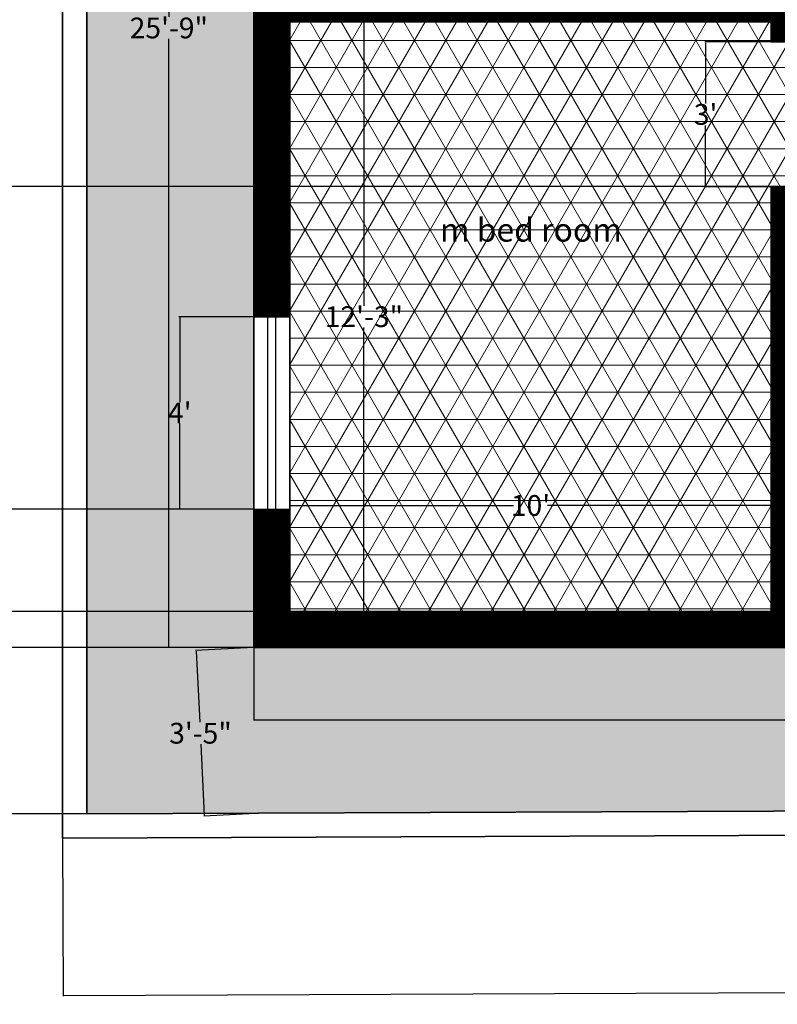
# Model space of a CAD drawing. Units: inches. Extents: x -157 to 1464, y -361 to 1077.
# Tile 3 of 9: x 241 to 430, y 23 to 268. Entities that reach past the tile are written whole.
import ezdxf

# ---------------------------------------------------------------- set-up
doc = ezdxf.new("R2010")
doc.units = ezdxf.units.IN
doc.header["$MEASUREMENT"] = 0
for name, color, linetype, lineweight in [('A-ANNO-DIMS', 2, 'Continuous', 18), ('A-AREA-IDEN', 7, 'Continuous', 18), ('A-FLOR-PATT', 8, 'Continuous', 13), ('A-WALL', 7, 'Continuous', 35), ('A-WALL-PATT', 252, 'Continuous', 13), ('C-ANNO-DIMS', 2, 'Continuous', 18), ('C-PROP', 7, 'Continuous', 35), ('doors and windows', 33, 'Continuous', 25), ('L-GRND-PATT', 8, 'Continuous', 13)]:
    doc.layers.add(name, color=color, linetype=linetype, lineweight=lineweight)
doc.styles.get("Standard").update_dxf_attribs({"font": 'arial.ttf'})
doc.dimstyles.new('Annotative', dxfattribs={"dimscale": 0, "dimtxt": 5.18, "dimasz": 0.18, "dimexe": 0.18, "dimexo": 0.0625, "dimgap": 0.09, "dimtad": 0, "dimtih": 1, "dimtoh": 1, "dimdec": 0, "dimzin": 0, "dimdsep": 46, "dimlunit": 3, "dimtxsty": 'Standard', "dimcen": 0.09, "dimadec": 0, "dimazin": 0, "dimtfac": 1, "dimtdec": 0, "dimtofl": 0, "dimtmove": 0, "dimatfit": 3, "dimfxl": 1, "dimtolj": 1, "dimtzin": 0, "dimarcsym": 0})

# ---------------------------------------------------------------- blocks, each defined once
blk = doc.blocks.new('*D1')
at = {"layer": 'A-ANNO-DIMS', "color": 0, "lineweight": -2, "transparency": 16777216}
for p, q in [((298.9, 420.86), (277.62, 420.86)), ((277.8, 420.68), (277.8, 269.1)), ((277.8, 112.04), (277.8, 263.63)), ((298.9, 111.86), (277.62, 111.86))]:
    blk.add_line(p, q, dxfattribs=at)
at = {"layer": 'A-ANNO-DIMS', "color": 0, "transparency": 16777216}
for points in [[(277.77, 420.68), (277.83, 420.68), (277.8, 420.86)], [(277.77, 112.04), (277.83, 112.04), (277.8, 111.86)]]:
    blk.add_solid(points, dxfattribs=at)
at = {"layer": 'Defpoints', "color": 0, "transparency": 16777216}
for p in [(298.97, 420.86), (277.8, 111.86), (298.97, 111.86)]:
    blk.add_point(p, dxfattribs=at)
at = {"layer": 'A-ANNO-DIMS', "color": 0, "transparency": 16777216, "insert": (277.8, 266.36), "char_height": 5.18, "attachment_point": 5}
blk.add_mtext('\\A1;25\'-9"', dxfattribs=at)
blk = doc.blocks.new('*D2')
at = {"layer": 'A-ANNO-DIMS', "color": 0, "lineweight": -2, "transparency": 16777216}
for p, q in [((298.97, 111.8), (298.97, 93.67)), ((596.97, 111.8), (596.97, 93.67)), ((299.15, 93.85), (436.92, 93.85)), ((596.79, 93.85), (459.01, 93.85))]:
    blk.add_line(p, q, dxfattribs=at)
at = {"layer": 'A-ANNO-DIMS', "color": 0, "transparency": 16777216}
for points in [[(299.15, 93.88), (299.15, 93.82), (298.97, 93.85)], [(596.79, 93.88), (596.79, 93.82), (596.97, 93.85)]]:
    blk.add_solid(points, dxfattribs=at)
at = {"layer": 'Defpoints', "color": 0, "transparency": 16777216}
for p in [(298.97, 111.86), (596.97, 111.86), (596.97, 93.85)]:
    blk.add_point(p, dxfattribs=at)
at = {"layer": 'A-ANNO-DIMS', "color": 0, "transparency": 16777216, "insert": (447.97, 93.85), "char_height": 5.18, "attachment_point": 5}
blk.add_mtext('\\A1;24\'-10"', dxfattribs=at)
blk = doc.blocks.new('*D3')
at = {"layer": 'A-ANNO-DIMS', "color": 0, "lineweight": -2, "transparency": 16777216}
for p, q in [((308.03, 267.86), (326.61, 267.86)), ((326.43, 267.68), (326.43, 197.1)), ((326.43, 121.04), (326.43, 191.62)), ((308.03, 120.86), (326.61, 120.86))]:
    blk.add_line(p, q, dxfattribs=at)
at = {"layer": 'A-ANNO-DIMS', "color": 0, "transparency": 16777216}
for points in [[(326.4, 267.68), (326.46, 267.68), (326.43, 267.86)], [(326.4, 121.04), (326.46, 121.04), (326.43, 120.86)]]:
    blk.add_solid(points, dxfattribs=at)
at = {"layer": 'Defpoints', "color": 0, "transparency": 16777216}
for p in [(307.97, 267.86), (307.97, 120.86), (326.43, 120.86)]:
    blk.add_point(p, dxfattribs=at)
at = {"layer": 'A-ANNO-DIMS', "color": 0, "transparency": 16777216, "insert": (326.43, 194.36), "char_height": 5.18, "attachment_point": 5}
blk.add_mtext('\\A1;12\'-3"', dxfattribs=at)
blk = doc.blocks.new('*D4')
at = {"layer": 'A-ANNO-DIMS', "color": 0, "lineweight": -2, "transparency": 16777216}
for p, q in [((307.97, 120.92), (307.97, 147.45)), ((427.97, 120.92), (427.97, 147.45)), ((308.15, 147.27), (363.72, 147.27)), ((427.79, 147.27), (372.21, 147.27))]:
    blk.add_line(p, q, dxfattribs=at)
at = {"layer": 'A-ANNO-DIMS', "color": 0, "transparency": 16777216}
for points in [[(308.15, 147.3), (308.15, 147.24), (307.97, 147.27)], [(427.79, 147.3), (427.79, 147.24), (427.97, 147.27)]]:
    blk.add_solid(points, dxfattribs=at)
at = {"layer": 'Defpoints', "color": 0, "transparency": 16777216}
for p in [(427.97, 147.27), (307.97, 120.86), (427.97, 120.86)]:
    blk.add_point(p, dxfattribs=at)
at = {"layer": 'A-ANNO-DIMS', "color": 0, "transparency": 16777216, "insert": (367.97, 147.27), "char_height": 5.18, "attachment_point": 5}
blk.add_mtext("\\A1;10'", dxfattribs=at)
blk = doc.blocks.new('*D13')
at = {"layer": 'C-ANNO-DIMS', "color": 0, "lineweight": -2, "transparency": 16777216}
for p, q in [((257.27, 643.42), (188.08, 643.42)), ((188.26, 643.24), (188.26, 359.63)), ((188.26, 70.55), (188.26, 354.16)), ((257.27, 70.37), (188.08, 70.37))]:
    blk.add_line(p, q, dxfattribs=at)
at = {"layer": 'C-ANNO-DIMS', "color": 0, "transparency": 16777216}
for points in [[(188.23, 643.24), (188.29, 643.24), (188.26, 643.42)], [(188.23, 70.55), (188.29, 70.55), (188.26, 70.37)]]:
    blk.add_solid(points, dxfattribs=at)
at = {"layer": 'Defpoints', "color": 0, "transparency": 16777216}
for p in [(257.33, 643.42), (188.26, 70.37), (257.33, 70.37)]:
    blk.add_point(p, dxfattribs=at)
at = {"layer": 'C-ANNO-DIMS', "color": 0, "transparency": 16777216, "insert": (188.26, 356.89), "char_height": 5.18, "attachment_point": 5}
blk.add_mtext('\\A1;47\'-9"', dxfattribs=at)
blk = doc.blocks.new('*D14')
at = {"layer": 'C-ANNO-DIMS', "color": 0, "lineweight": -2, "transparency": 16777216}
for p, q in [((862.57, 66.62), (862.72, 27.26)), ((251.33, 64.28), (251.48, 24.92)), ((862.54, 27.44), (568.1, 26.31)), ((251.66, 25.1), (546.1, 26.23))]:
    blk.add_line(p, q, dxfattribs=at)
at = {"layer": 'C-ANNO-DIMS', "color": 0, "transparency": 16777216}
for points in [[(862.54, 27.47), (862.54, 27.41), (862.72, 27.44)], [(251.66, 25.13), (251.66, 25.07), (251.48, 25.1)]]:
    blk.add_solid(points, dxfattribs=at)
at = {"layer": 'Defpoints', "color": 0, "transparency": 16777216}
for p in [(862.57, 66.68), (251.33, 64.34), (862.72, 27.44)]:
    blk.add_point(p, dxfattribs=at)
at = {"layer": 'C-ANNO-DIMS', "color": 0, "transparency": 16777216, "insert": (557.1, 26.27), "char_height": 5.18, "attachment_point": 5}
blk.add_mtext('\\A1;50\'-11"', dxfattribs=at)
blk = doc.blocks.new('*D28')
at = {"layer": 'A-ANNO-DIMS', "color": 0, "lineweight": -2, "transparency": 16777216}
for p, q in [((427.9, 262.86), (411.45, 262.86)), ((411.63, 262.68), (411.63, 247.54)), ((411.63, 226.92), (411.63, 242.06)), ((427.9, 226.74), (411.45, 226.74))]:
    blk.add_line(p, q, dxfattribs=at)
at = {"layer": 'A-ANNO-DIMS', "color": 0, "transparency": 16777216}
for points in [[(411.6, 262.68), (411.66, 262.68), (411.63, 262.86)], [(411.6, 226.92), (411.66, 226.92), (411.63, 226.74)]]:
    blk.add_solid(points, dxfattribs=at)
at = {"layer": 'Defpoints', "color": 0, "transparency": 16777216}
for p in [(427.97, 262.86), (411.63, 226.74), (427.97, 226.74)]:
    blk.add_point(p, dxfattribs=at)
at = {"layer": 'A-ANNO-DIMS', "color": 0, "transparency": 16777216, "insert": (411.63, 244.8), "char_height": 5.18, "attachment_point": 5}
blk.add_mtext("\\A1;3'", dxfattribs=at)
blk = doc.blocks.new('*D49')
at = {"layer": 'A-ANNO-DIMS', "color": 0, "lineweight": -2, "transparency": 16777216}
for p, q in [((298.9, 194.36), (280.34, 194.36)), ((280.52, 194.18), (280.52, 173.04)), ((280.52, 146.54), (280.52, 167.68)), ((298.9, 146.36), (280.34, 146.36))]:
    blk.add_line(p, q, dxfattribs=at)
at = {"layer": 'A-ANNO-DIMS', "color": 0, "transparency": 16777216}
for points in [[(280.49, 194.18), (280.55, 194.18), (280.52, 194.36)], [(280.49, 146.54), (280.55, 146.54), (280.52, 146.36)]]:
    blk.add_solid(points, dxfattribs=at)
at = {"layer": 'Defpoints', "color": 0, "transparency": 16777216}
for p in [(298.97, 194.36), (280.52, 146.36), (298.97, 146.36)]:
    blk.add_point(p, dxfattribs=at)
at = {"layer": 'A-ANNO-DIMS', "color": 0, "transparency": 16777216, "insert": (280.52, 170.36), "char_height": 5.18, "attachment_point": 5}
blk.add_mtext("\\A1;4'", dxfattribs=at)
blk = doc.blocks.new('*D54')
at = {"layer": 'C-ANNO-DIMS', "color": 0, "lineweight": -2, "transparency": 16777216}
for p, q in [((298.9, 111.86), (284.47, 111.13)), ((284.66, 110.96), (285.56, 93.21)), ((286.74, 69.99), (285.84, 87.73)), ((301, 70.53), (286.57, 69.8))]:
    blk.add_line(p, q, dxfattribs=at)
at = {"layer": 'C-ANNO-DIMS', "color": 0, "transparency": 16777216}
for points in [[(284.69, 110.96), (284.63, 110.95), (284.65, 111.14)], [(286.77, 69.99), (286.71, 69.99), (286.75, 69.81)]]:
    blk.add_solid(points, dxfattribs=at)
at = {"layer": 'Defpoints', "color": 0, "transparency": 16777216}
for p in [(298.97, 111.86), (286.75, 69.81), (301.06, 70.53)]:
    blk.add_point(p, dxfattribs=at)
at = {"layer": 'C-ANNO-DIMS', "color": 0, "transparency": 16777216, "insert": (285.7, 90.47), "char_height": 5.18, "attachment_point": 5}
blk.add_mtext('\\A1;3\'-5"', dxfattribs=at)
blk = doc.blocks.new('WIN-48x9')
for p, q in [((9, 48), (0, 48)), ((0, 48), (0, 0)), ((3.5, 48), (3.5, 0)), ((5.5, 48), (5.5, 0)), ((9, 48), (9, 0)), ((9, 0), (0, 0))]:
    blk.add_line(p, q)
blk = doc.blocks.new('*D71')
at = {"layer": 'A-ANNO-DIMS', "color": 0, "lineweight": -2, "transparency": 16777216}
for p, q in [((298.9, 146.36), (-141.39, 146.36)), ((-141.21, 146.18), (-141.21, 131.88)), ((-141.21, 112.04), (-141.21, 126.34)), ((298.9, 111.86), (-141.39, 111.86))]:
    blk.add_line(p, q, dxfattribs=at)
at = {"layer": 'A-ANNO-DIMS', "color": 0, "transparency": 16777216}
for points in [[(-141.24, 146.18), (-141.18, 146.18), (-141.21, 146.36)], [(-141.24, 112.04), (-141.18, 112.04), (-141.21, 111.86)]]:
    blk.add_solid(points, dxfattribs=at)
at = {"layer": 'Defpoints', "color": 0, "transparency": 16777216}
for p in [(-141.21, 146.36), (298.97, 146.36), (298.97, 111.86)]:
    blk.add_point(p, dxfattribs=at)
at = {"layer": 'A-ANNO-DIMS', "color": 0, "transparency": 16777216, "insert": (-141.21, 129.11), "char_height": 5.18, "attachment_point": 5}
blk.add_mtext('\\A1;2\'-10 1/2"', dxfattribs=at)
blk = doc.blocks.new('*D78')
at = {"layer": 'A-ANNO-DIMS', "color": 0, "lineweight": -2, "transparency": 16777216}
for p, q in [((427.9, 226.86), (-141.39, 226.86)), ((-141.21, 226.68), (-141.21, 176.6)), ((-141.21, 121.04), (-141.21, 171.13)), ((427.9, 120.86), (-141.39, 120.86))]:
    blk.add_line(p, q, dxfattribs=at)
at = {"layer": 'A-ANNO-DIMS', "color": 0, "transparency": 16777216}
for points in [[(-141.24, 226.68), (-141.18, 226.68), (-141.21, 226.86)], [(-141.24, 121.04), (-141.18, 121.04), (-141.21, 120.86)]]:
    blk.add_solid(points, dxfattribs=at)
at = {"layer": 'Defpoints', "color": 0, "transparency": 16777216}
for p in [(427.97, 226.86), (-141.21, 120.86), (427.97, 120.86)]:
    blk.add_point(p, dxfattribs=at)
at = {"layer": 'A-ANNO-DIMS', "color": 0, "transparency": 16777216, "insert": (-141.21, 173.86), "char_height": 5.18, "attachment_point": 5}
blk.add_mtext('\\A1;8\'-10"', dxfattribs=at)

msp = doc.modelspace()

# ---------------------------------------------------------------- hatches: boundary and pattern name
at = {"layer": 'A-FLOR-PATT'}
h = msp.add_hatch(dxfattribs=at)
h.set_pattern_fill('NET3', color=256, scale=54)
h.paths.add_polyline_path([(563.97, 267.86), (480.97, 267.86), (480.97, 272.86), (432.97, 272.86), (432.97, 262.86), (427.97, 262.86), (427.97, 267.86), (307.97, 267.86), (307.97, 120.86), (427.97, 120.86), (427.97, 226.86), (432.97, 226.86), (432.97, 203.86), (438.97, 203.86), (468.97, 203.86), (485.97, 203.86), (485.97, 144.86), (563.97, 144.86)])
h.paths.add_polyline_path([(507.66, 186.06), (540.97, 186.06), (540.97, 198.1), (507.66, 198.1)], flags=24)
h.paths.add_polyline_path([(343.4, 209.88), (389.84, 209.88), (389.84, 221.92), (343.4, 221.92)], flags=24)
at = {"layer": 'A-WALL-PATT'}
h = msp.add_hatch(dxfattribs=at)
h.set_pattern_fill('ANSI31', color=256)
h.set_pattern_definition([(45, (213.19381, 103.60139), (-0.088388348, 0.088388348), [])])
h.paths.add_polyline_path([(307.97, 267.86), (427.97, 267.86), (427.97, 262.86), (432.97, 262.86), (432.97, 277.86), (427.97, 277.86), (427.97, 272.86), (307.97, 272.86), (307.97, 276.53), (298.97, 276.53), (298.97, 194.36), (307.97, 194.36)])
h.paths.add_polyline_path([(307.97, 411.86), (427.97, 411.86), (427.97, 313.86), (432.97, 313.86), (432.97, 411.86), (463.95, 411.86), (463.95, 420.86), (298.97, 420.86), (298.97, 324.53), (307.97, 324.53)])
h.paths.add_polyline_path([(511.95, 420.86), (511.95, 411.86), (546.97, 411.86), (546.97, 420.86)])
h.paths.add_polyline_path([(587.97, 411.86), (587.97, 405.86), (596.97, 405.86), (596.97, 420.86), (582.97, 420.86), (582.97, 411.86)])
h.paths.add_polyline_path([(587.97, 369.86), (587.97, 324), (596.97, 324), (596.97, 369.86)])
h.paths.add_polyline_path([(596.97, 276), (587.97, 276), (587.97, 272.86), (480.97, 272.86), (480.97, 267.86), (587.97, 267.86), (587.97, 206.9), (596.97, 206.9)])
h.paths.add_polyline_path([(587.97, 120.86), (485.97, 120.86), (485.97, 203.86), (468.97, 203.86), (468.97, 198.86), (480.97, 198.86), (480.97, 120.86), (465.97, 120.86), (465.97, 111.86), (596.97, 111.86), (596.97, 158.9), (587.97, 158.9)])
h.paths.add_polyline_path([(427.97, 120.86), (307.97, 120.86), (307.97, 146.36), (298.97, 146.36), (298.97, 111.86), (447.97, 111.86), (447.97, 120.86), (432.97, 120.86), (432.97, 198.86), (438.97, 198.86), (438.97, 203.86), (432.97, 203.86), (432.97, 226.86), (427.97, 226.86)])
at = {"layer": 'L-GRND-PATT'}
h = msp.add_hatch(dxfattribs=at)
h.set_pattern_fill('GRAVEL', color=256, scale=26)
h.set_pattern_definition([(228.01279, (18.72, 26), (-208, -234), [3.49794, -346.2963]), (184.96974, (16.38, 23.4), (312, 26), [6.00257, -594.25404]), (132.51045, (10.4, 22.88), (260, -286), [4.2325, -419.01685]), (267.27369, (0.26, 16.38), (26, 520), [5.4662, -541.1525]), (292.83365, (0, 10.92), (-130, 312), [5.36003, -530.6437]), (357.27369, (2.08, 5.98), (-520, 26), [5.4662, -541.1525]), (37.69424, (7.54, 5.72), (-338, -260), [7.22875, -715.64606]), (72.25533, (13.26, 10.14), (182, 572), [6.8247, -675.64436]), (121.42957, (15.34, 16.64), (-208, 338), [5.4847, -542.9859]), (175.23636, (12.48, 21.32), (286, -26), [6.26163, -306.81983]), (222.39744, (6.24, 21.84), (-312, -286), [8.09765, -801.66775]), (138.81407, (26, 16.12), (-182, 156), [2.76383, -273.61997]), (171.46923, (23.92, 17.94), (338, -52), [5.25816, -520.5593]), (225, (18.72, 18.72), (-3e-15, -26), [3.67695, -33.0926]), (203.1986, (16.9, 21.84), (130, 52), [1.9801, -196.03]), (291.8014, (15.08, 21.06), (-26, 78), [2.8003, -137.214]), (30.96376, (16.12, 18.46), (78, 52), [4.54815, -147.0566]), (161.56505, (20.02, 20.8), (52, -26), [3.28877, -78.93045]), (16.38954, (0, 21.06), (260, 78), [4.6072, -456.11397]), (70.34618, (4.42, 22.36), (-104, -286), [3.8652, -382.6526]), (293.1986, (20.02, 26), (-52, 130), [3.9602, -194.0499]), (343.61046, (21.58, 22.36), (-260, 78), [4.6072, -456.11397]), (339.44395, (0, 4.94), (-130, 52), [4.4429, -217.7012]), (294.77514, (4.16, 3.38), (-130, 286), [3.72263, -368.5407]), (66.8014, (20.28, 0), (52, 130), [3.9602, -194.0499]), (17.35402, (21.84, 3.64), (-338, -104), [4.3584, -431.481]), (69.44395, (7.54, 0), (-52, -130), [2.22144, -219.92266]), (101.30993, (18.72, 0), (-26, 104), [1.32574, -131.24877]), (165.96376, (18.46, 1.3), (78, -26), [5.36003, -101.8407]), (186.009, (13.26, 2.6), (260, 26), [4.9673, -491.762]), (303.6901, (16.12, 16.12), (-26, 52), [3.7498, -89.99456]), (353.15723, (18.2, 13), (442, -52), [6.54664, -648.11663]), (60.9454, (24.7, 12.22), (-104, -182), [2.67686, -265.00953]), (90, (26, 14.56), (-26, 26), [1.56, -24.44]), (120.25644, (12.74, 3.38), (104, -182), [3.61202, -357.5915]), (48.01279, (10.92, 6.5), (208, 234), [6.99587, -342.79835]), (0, (15.6, 11.7), (26, 26), [6.76, -19.24]), (325.30485, (22.36, 11.7), (260, -182), [4.11096, -406.98513]), (254.0546, (25.74, 9.36), (-26, -104), [3.78565, -185.4972]), (207.64598, (24.7, 5.72), (-494, -260), [6.1637, -610.20633]), (175.42608, (19.24, 2.86), (-338, 26), [6.52077, -645.5559])])
h.paths.add_polyline_path([(856.57, 645.71), (257.33, 643.42), (257.33, 70.37), (856.57, 72.66)])
h.paths.add_polyline_path([(668.97, 111.86), (596.97, 111.86), (298.97, 111.86), (298.97, 420.86), (298.97, 492.86), (427.97, 492.86), (668.97, 492.86)], flags=16)
h.paths.add_polyline_path([(842.44, 305.24), (842.44, 199.78), (692.18, 199.78), (692.18, 305.24)], flags=16)
h.paths.add_polyline_path([(596.97, 369.86), (596.97, 158.9), (587.97, 158.9), (587.97, 120.86), (485.97, 120.86), (485.97, 203.86), (468.97, 203.86), (468.97, 198.86), (480.97, 198.86), (480.97, 120.86), (465.97, 120.86), (465.97, 111.86), (447.97, 111.86), (447.97, 120.86), (432.97, 120.86), (432.97, 198.86), (438.97, 198.86), (438.97, 203.86), (432.97, 203.86), (432.97, 226.86), (427.97, 226.86), (427.97, 120.86), (307.97, 120.86), (307.97, 146.36), (298.97, 146.36), (298.97, 194.36), (307.97, 194.36), (307.97, 267.86), (427.97, 267.86), (427.97, 262.86), (432.97, 262.86), (432.97, 277.86), (427.97, 277.86), (427.97, 272.86), (307.97, 272.86), (307.97, 276.53), (298.97, 276.53), (298.97, 324.53), (307.97, 324.53), (307.97, 411.86), (427.97, 411.86), (427.97, 313.86), (432.97, 313.86), (432.97, 411.86), (463.95, 411.86), (463.95, 420.86), (334.97, 420.86), (334.97, 456.86), (427.97, 456.86), (427.97, 420.86), (546.97, 420.86), (582.97, 420.86), (596.97, 420.86), (596.97, 405.86)], flags=0)
h.paths.add_polyline_path([(596.97, 369.86), (587.97, 369.86), (587.97, 324), (596.97, 324), (596.97, 276), (587.97, 276), (587.97, 369.86), (587.97, 405.86), (587.97, 411.86), (582.97, 411.86), (546.97, 411.86), (546.97, 420.86), (564.97, 416.36), (582.97, 420.86), (582.97, 411.86), (587.97, 411.86), (587.97, 405.86), (596.97, 405.86), (592.47, 387.86)], flags=0)
h.paths.add_polyline_path([(468.97, 203.86), (468.97, 198.86), (438.97, 198.86), (438.97, 203.86)], flags=0)
h.paths.add_polyline_path([(267.35, 260.99), (288.37, 260.99), (288.37, 271.66), (267.35, 271.66)], flags=24)
h.paths.add_polyline_path([(435.51, 88.48), (460.55, 88.48), (460.55, 99.15), (435.51, 99.15)], flags=24)
h.paths.add_polyline_path([(315.69, 188.99), (336.72, 188.99), (336.72, 199.66), (315.69, 199.66)], flags=8)
h.paths.add_polyline_path([(361.73, 141.9), (373.75, 141.9), (373.75, 152.57), (361.73, 152.57)], flags=8)
h.paths.add_polyline_path([(430.38, 154.49), (447.38, 154.49), (447.38, 165.16), (430.38, 165.16)], flags=8)
h.paths.add_polyline_path([(451.09, 165.32), (468.09, 165.32), (468.09, 175.99), (451.09, 175.99)], flags=8)
h.paths.add_polyline_path([(361.73, 305.06), (373.75, 305.06), (373.75, 315.74), (361.73, 315.74)], flags=8)
h.paths.add_polyline_path([(316.13, 336.94), (337.15, 336.94), (337.15, 347.62), (316.13, 347.62)], flags=8)
h.paths.add_polyline_path([(484.07, 423.56), (492.07, 423.56), (492.07, 434.24), (484.07, 434.24)], flags=8)
h.paths.add_polyline_path([(560.99, 428.52), (568.98, 428.52), (568.98, 439.19), (560.99, 439.19)], flags=8)
h.paths.add_polyline_path([(528.49, 131.95), (545.49, 131.95), (545.49, 142.62), (528.49, 142.62)], flags=8)
h.paths.add_polyline_path([(564.53, 188.99), (585.55, 188.99), (585.55, 199.66), (564.53, 199.66)], flags=8)

# ---------------------------------------------------------------- linework, layer by layer
at = {"layer": 'A-WALL'}
for p, q in [((298.97, 111.86), (298.97, 420.86)), ((307.97, 120.86), (307.97, 267.86)), ((307.97, 267.86), (427.97, 267.86)), ((427.97, 262.86), (427.97, 267.86)), ((427.97, 262.86), (432.97, 262.86)), ((427.97, 120.86), (427.97, 226.86)), ((427.97, 226.86), (432.97, 226.86)), ((427.97, 120.86), (307.97, 120.86)), ((596.97, 111.86), (298.97, 111.86))]:
    msp.add_line(p, q, dxfattribs=at)
at = {"layer": 'C-PROP'}
msp.add_lwpolyline([(862.57, 615.42), (862.57, 651.74), (251.33, 649.4), (251.33, 64.34), (862.57, 66.68), (862.57, 519.42)], dxfattribs=at)
msp.add_lwpolyline([(257.33, 70.37), (856.57, 72.66), (856.57, 645.71), (257.33, 643.42)], close=True, dxfattribs=at)

# ---------------------------------------------------------------- block references
at = {"layer": 'doors and windows', "rotation": 180}
msp.add_blockref('WIN-48x9', (307.97, 194.36), dxfattribs=at)

# ---------------------------------------------------------------- texts
at = {"layer": 'A-AREA-IDEN', "insert": (345.4, 218.91), "char_height": 5.84, "attachment_point": 1}
msp.add_mtext_dynamic_manual_height_columns('m bed room', width=87.358, gutter_width=29.2, heights=[13.12], dxfattribs=at)

# ---------------------------------------------------------------- dimensions: what is measured, and where the dimension line sits
at = {"layer": 'A-ANNO-DIMS'}
for base, p1, p2, override, picture, middle in [((277.8, 111.86), (298.97, 420.86), (298.97, 111.86), {"dimclrd": 0, "dimclre": 0, "dimclrt": 0}, '*D1', (277.8, 266.36)), ((411.63, 226.74), (427.97, 262.86), (427.97, 226.74), {"dimclrd": 0, "dimclre": 0, "dimclrt": 0}, '*D28', (411.63, 244.8)), ((-141.21, 120.86), (427.97, 226.86), (427.97, 120.86), {"dimscale": 1, "dimdec": 1, "dimzin": 1, "dimlunit": 4, "dimfrac": 2}, '*D78', (-141.21, 173.86)), ((280.52, 146.36), (298.97, 194.36), (298.97, 146.36), {"dimclrd": 0, "dimclre": 0, "dimclrt": 0}, '*D49', (280.52, 170.36)), ((-141.21, 146.36), (298.97, 111.86), (298.97, 146.36), {"dimscale": 1, "dimdec": 1, "dimzin": 1, "dimlunit": 4, "dimfrac": 2}, '*D71', (-141.21, 129.11))]:
    dim = msp.add_linear_dim(base=base, p1=p1, p2=p2, angle=90, dimstyle='Annotative', override=override, dxfattribs=at)
    dim.commit()
    dim.dimension.update_dxf_attribs({"geometry": picture, "text_midpoint": middle})
dim = msp.add_aligned_dim(p1=(307.97, 267.86), p2=(307.97, 120.86), distance=18.46, dimstyle='Annotative', override={"dimclrd": 0, "dimclre": 0, "dimclrt": 0}, dxfattribs=at)
dim.commit()
dim.dimension.update_dxf_attribs({"geometry": '*D3', "text_midpoint": (326.43, 194.36)})
for base, p1, p2, picture, middle in [((427.97, 147.27), (307.97, 120.86), (427.97, 120.86), '*D4', (367.97, 147.27)), ((596.97, 93.85), (298.97, 111.86), (596.97, 111.86), '*D2', (447.97, 93.85))]:
    dim = msp.add_linear_dim(base=base, p1=p1, p2=p2, dimstyle='Annotative', override={"dimclrd": 0, "dimclre": 0, "dimclrt": 0}, dxfattribs=at)
    dim.commit()
    dim.dimension.update_dxf_attribs({"geometry": picture, "text_midpoint": middle})
at = {"layer": 'C-ANNO-DIMS'}
dim = msp.add_linear_dim(base=(188.26, 70.37), p1=(257.33, 643.42), p2=(257.33, 70.37), angle=90, dimstyle='Annotative', override={"dimclrd": 0, "dimclre": 0, "dimclrt": 0}, dxfattribs=at)
dim.commit()
dim.dimension.update_dxf_attribs({"geometry": '*D13', "text_midpoint": (188.26, 356.89)})
for p1, p2, distance, picture, middle in [((298.97, 111.86), (301.06, 70.53), -14.33, '*D54', (285.7, 90.47)), ((251.33, 64.34), (862.57, 66.68), -39.24, '*D14', (557.1, 26.27))]:
    dim = msp.add_aligned_dim(p1=p1, p2=p2, distance=distance, dimstyle='Annotative', override={"dimclrd": 0, "dimclre": 0, "dimclrt": 0}, dxfattribs=at)
    dim.commit()
    dim.dimension.update_dxf_attribs({"geometry": picture, "text_midpoint": middle})

doc.saveas('drawing.dxf')
